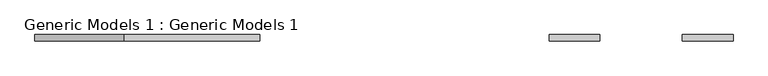
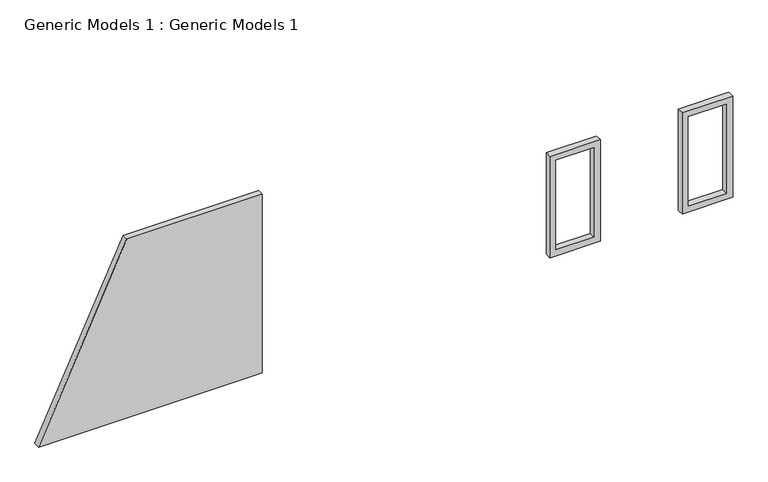
"""IFC4 building model written with IfcOpenShell, lengths in millimetres: proxy geometry, Generic Models 1 : Generic Models 1."""

from ifc_helpers import new_model, si_unit, frame, origin, place, context, project, spatial, polyline, outline, extrude, source, transform, mapped, element, save


def generic_models_1_generic_models_1_bb1f4732(model_context):
    return source(origin(), model_context, "Body", "SweptSolid", [
        extrude(outline(polyline([(1828.8, -543.1569651), (1828.8, -1635.3569651), (304.8, -2346.0098361), (304.8, -543.1569651), (1828.8, -543.1569651)])), frame((0.0, 400.7055142, 0.0), z_axis=(0.0, 1.0, 0.0), x_axis=(0.0, 0.0, 1.0)), (0.0, 0.0, 1.0), 50.8),
        extrude(outline(polyline([(1339.2781699, 2181.1534335), (1339.2781699, 1774.7534335), (475.6781699, 1774.7534335), (475.6781699, 2181.1534335), (1339.2781699, 2181.1534335)]), holes=[polyline([(1288.4781699, 2130.3534335), (526.4781699, 2130.3534335), (526.4781699, 1825.5534335), (1288.4781699, 1825.5534335), (1288.4781699, 2130.3534335)])]), frame((0.0, 400.7055142, 0.0), z_axis=(0.0, 1.0, 0.0), x_axis=(0.0, 0.0, 1.0)), (0.0, 0.0, 1.0), 50.8),
        extrude(outline(polyline([(1339.2781699, 3247.9534335), (1339.2781699, 2841.5534335), (475.6781699, 2841.5534335), (475.6781699, 3247.9534335), (1339.2781699, 3247.9534335)]), holes=[polyline([(1288.4781699, 3197.1534335), (526.4781699, 3197.1534335), (526.4781699, 2892.3534335), (1288.4781699, 2892.3534335), (1288.4781699, 3197.1534335)])]), frame((0.0, 400.7055142, 0.0), z_axis=(0.0, 1.0, 0.0), x_axis=(0.0, 0.0, 1.0)), (0.0, 0.0, 1.0), 50.8),
    ])


if __name__ == "__main__":
    model = new_model("IFC4")
    model_context = context("Model", 3, world=origin())
    ifc_project = project(units=[si_unit("LENGTHUNIT", "METRE", prefix="MILLI")], contexts=[model_context])
    site = spatial("IfcSite", under=ifc_project)
    building = spatial("IfcBuilding", under=site)
    placement = place(None, origin())
    generic_models_1_generic_models_1_shape = generic_models_1_generic_models_1_bb1f4732(model_context)
    element("IfcBuildingElementProxy", 1, Name="Generic Models 1 : Generic Models 1", ObjectType="Generic Models 1 : Generic Models 1", at=placement, inside=building, context=model_context, shape_type="MappedRepresentation", body=[
        mapped(generic_models_1_generic_models_1_shape, transform((0.0, 0.0, 0.0), x_axis=(1.0, 0.0, 0.0), y_axis=(0.0, 1.0, 0.0), z_axis=(0.0, 0.0, 1.0))),
    ])
    save(model, "model.ifc")

# Revit data of these elements
# Element 1 (IfcBuildingElementProxy, "Generic Models 1 : Generic Models 1")
#   Materials on its faces: "1 wood", "1 wall brown"
# Materials
#   "1 wood": class "Generic", colour RGB 120 120 120, transparency 0, Cost = 0
#   "1 wall brown": class "Generic", colour RGB 61 46 37, transparency 0, Cost = 0
